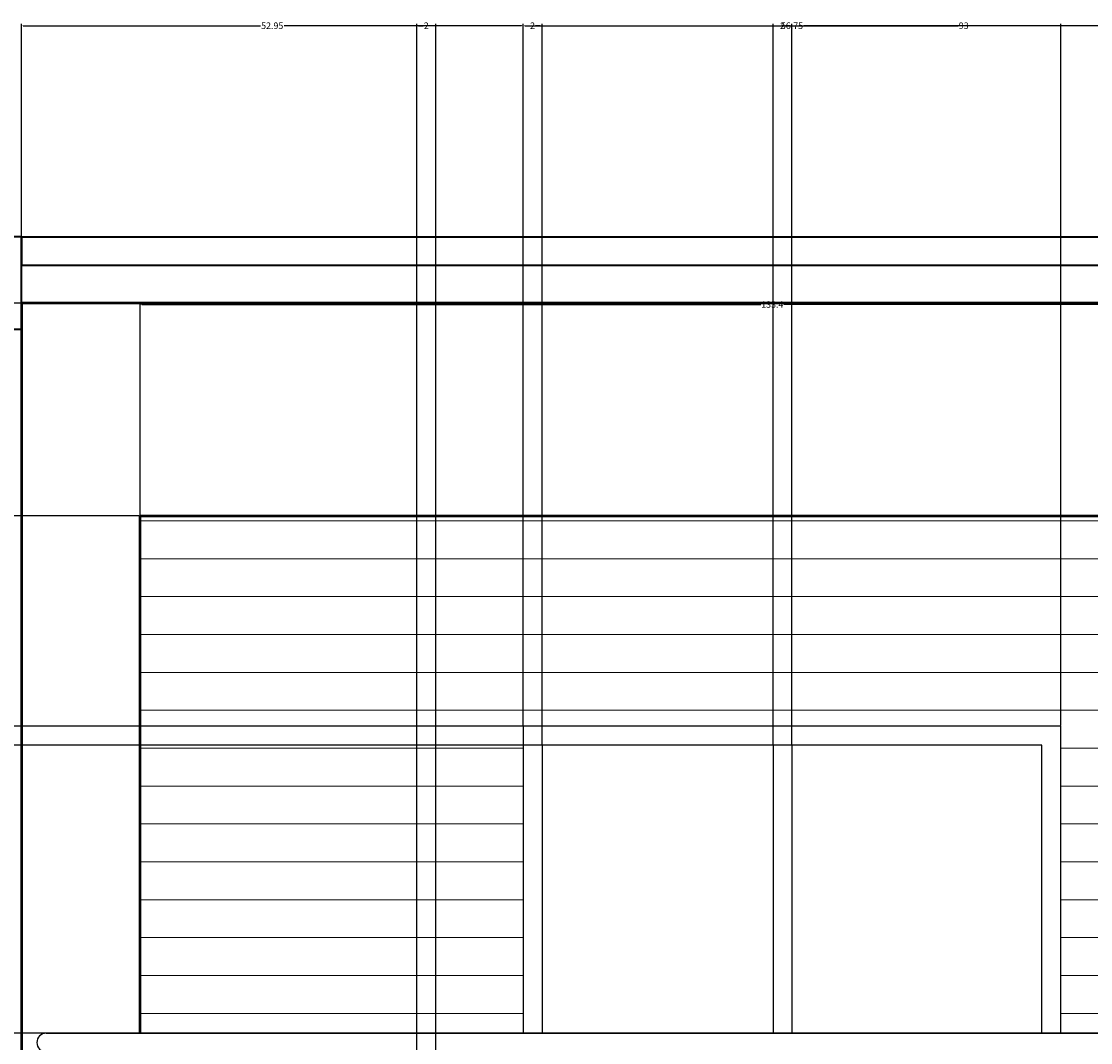
# Model space of a CAD drawing. Units: inches. Extents: x -139 to 346, y 72 to 413.
# Tile 8 of 18: x -47 to 66, y 305 to 413. Entities that reach past the tile are written whole.
import ezdxf

# ---------------------------------------------------------------- set-up
doc = ezdxf.new("R2010")
doc.units = ezdxf.units.IN
doc.header["$MEASUREMENT"] = 0
for name, color, linetype, lineweight in [('A-ANNO-DIMS', 2, 'Continuous', 18), ('A-DOOR', 3, 'Continuous', 25), ('A-ELEV-RAIL', 6, 'Continuous', 25), ('A-ROOF', 1, 'Continuous', 35), ('A-WALL', 7, 'Continuous', 50), ('A-WALL-PATT', 8, 'Continuous', 13)]:
    doc.layers.add(name, color=color, linetype=linetype, lineweight=lineweight)
doc.styles.get("Standard").update_dxf_attribs({"font": 'arial.ttf'})
doc.dimstyles.get("Standard").update_dxf_attribs({"dimtxt": 0.6875, "dimasz": 0.18, "dimexe": 0.18, "dimexo": 0.0625, "dimgap": 0.09, "dimtad": 0, "dimtih": 1, "dimtoh": 1, "dimdec": 4, "dimzin": 0, "dimdsep": 46, "dimlunit": 4, "dimtxsty": 'Standard', "dimcen": 0.09, "dimadec": 0, "dimazin": 0, "dimtfac": 1, "dimtdec": 4, "dimtofl": 0, "dimtmove": 0, "dimatfit": 3, "dimfxl": 1, "dimtolj": 1, "dimtzin": 0, "dimarcsym": 0})

# ---------------------------------------------------------------- blocks, each defined once
blk = doc.blocks.new('*D23')
at = {"layer": 'A-ANNO-DIMS', "color": 0, "lineweight": -2, "transparency": 16777216}
for p, q in [((-47.27, 383.04), (-47.27, 412.45)), ((-47.09, 412.27), (-22.05, 412.27)), ((5.49, 412.27), (-19.55, 412.27)), ((5.67, 338.38), (5.67, 412.45))]:
    blk.add_line(p, q, dxfattribs=at)
at = {"layer": 'A-ANNO-DIMS', "color": 0, "transparency": 16777216}
for points in [[(-47.09, 412.3), (-47.09, 412.24), (-47.27, 412.27)], [(5.49, 412.3), (5.49, 412.24), (5.67, 412.27)]]:
    blk.add_solid(points, dxfattribs=at)
at = {"layer": 'Defpoints', "color": 0, "transparency": 16777216}
for p in [(5.67, 412.27), (-47.27, 382.97), (5.67, 338.32)]:
    blk.add_point(p, dxfattribs=at)
at = {"layer": 'A-ANNO-DIMS', "color": 0, "transparency": 16777216, "insert": (-20.8, 412.27), "char_height": 0.688, "attachment_point": 5}
blk.add_mtext('\\A1;52.95', dxfattribs=at)
blk = doc.blocks.new('*D24')
at = {"layer": 'A-ANNO-DIMS', "color": 0, "lineweight": -2, "transparency": 16777216}
for p, q in [((5.67, 338.38), (5.67, 412.45)), ((5.85, 412.27), (32.8, 412.27)), ((62.25, 412.27), (35.3, 412.27)), ((62.43, 338.38), (62.43, 412.45))]:
    blk.add_line(p, q, dxfattribs=at)
at = {"layer": 'A-ANNO-DIMS', "color": 0, "transparency": 16777216}
for points in [[(5.85, 412.3), (5.85, 412.24), (5.67, 412.27)], [(62.25, 412.3), (62.25, 412.24), (62.43, 412.27)]]:
    blk.add_solid(points, dxfattribs=at)
at = {"layer": 'Defpoints', "color": 0, "transparency": 16777216}
for p in [(62.43, 412.27), (5.67, 338.32), (62.43, 338.32)]:
    blk.add_point(p, dxfattribs=at)
at = {"layer": 'A-ANNO-DIMS', "color": 0, "transparency": 16777216, "insert": (34.05, 412.27), "char_height": 0.688, "attachment_point": 5}
blk.add_mtext('\\A1;56.75', dxfattribs=at)
blk = doc.blocks.new('*D25')
at = {"layer": 'A-ANNO-DIMS', "color": 0, "lineweight": -2, "transparency": 16777216}
for p, q in [((5.67, 338.38), (5.67, 412.45)), ((5.85, 412.27), (51.59, 412.27)), ((98.49, 412.27), (52.76, 412.27)), ((98.67, 360.61), (98.67, 412.45))]:
    blk.add_line(p, q, dxfattribs=at)
at = {"layer": 'A-ANNO-DIMS', "color": 0, "transparency": 16777216}
for points in [[(5.85, 412.3), (5.85, 412.24), (5.67, 412.27)], [(98.49, 412.3), (98.49, 412.24), (98.67, 412.27)]]:
    blk.add_solid(points, dxfattribs=at)
at = {"layer": 'Defpoints', "color": 0, "transparency": 16777216}
for p in [(98.67, 412.27), (98.67, 360.54), (5.67, 338.32)]:
    blk.add_point(p, dxfattribs=at)
at = {"layer": 'A-ANNO-DIMS', "color": 0, "transparency": 16777216, "insert": (52.17, 412.27), "char_height": 0.688, "attachment_point": 5}
blk.add_mtext('\\A1;93', dxfattribs=at)
blk = doc.blocks.new('*D30')
at = {"layer": 'A-ANNO-DIMS', "color": 0, "lineweight": -2, "transparency": 16777216}
for p, q in [((-34.73, 360.61), (-34.73, 383.02)), ((-34.55, 382.84), (30.75, 382.84)), ((98.49, 382.84), (33.19, 382.84)), ((98.67, 360.61), (98.67, 383.02))]:
    blk.add_line(p, q, dxfattribs=at)
at = {"layer": 'A-ANNO-DIMS', "color": 0, "transparency": 16777216}
for points in [[(-34.55, 382.87), (-34.55, 382.81), (-34.73, 382.84)], [(98.49, 382.87), (98.49, 382.81), (98.67, 382.84)]]:
    blk.add_solid(points, dxfattribs=at)
at = {"layer": 'Defpoints', "color": 0, "transparency": 16777216}
for p in [(98.67, 382.84), (-34.73, 360.54), (98.67, 360.54)]:
    blk.add_point(p, dxfattribs=at)
at = {"layer": 'A-ANNO-DIMS', "color": 0, "transparency": 16777216, "insert": (31.97, 382.84), "char_height": 0.688, "attachment_point": 5}
blk.add_mtext('\\A1;133.4', dxfattribs=at)
blk = doc.blocks.new('*D44')
at = {"layer": 'A-ANNO-DIMS', "color": 0, "lineweight": -2, "transparency": 16777216}
for p, q in [((5.61, 338.32), (-137.3, 338.32)), ((-137.12, 338.14), (-137.12, 315.13)), ((-137.12, 291.24), (-137.12, 314.25)), ((-47.34, 291.06), (-137.3, 291.06))]:
    blk.add_line(p, q, dxfattribs=at)
at = {"layer": 'A-ANNO-DIMS', "color": 0, "transparency": 16777216}
for points in [[(-137.15, 338.14), (-137.09, 338.14), (-137.12, 338.32)], [(-137.15, 291.24), (-137.09, 291.24), (-137.12, 291.06)]]:
    blk.add_solid(points, dxfattribs=at)
at = {"layer": 'Defpoints', "color": 0, "transparency": 16777216}
for p in [(-137.12, 338.32), (5.67, 338.32), (-47.27, 291.06)]:
    blk.add_point(p, dxfattribs=at)
at = {"layer": 'A-ANNO-DIMS', "color": 0, "transparency": 16777216, "insert": (-137.12, 314.69), "char_height": 0.688, "attachment_point": 5}
blk.add_mtext('\\A1;47.26', dxfattribs=at)
blk = doc.blocks.new('*D45')
at = {"layer": 'A-ANNO-DIMS', "color": 0, "lineweight": -2, "transparency": 16777216}
for p, q in [((-34.8, 360.54), (-137.3, 360.54)), ((-137.12, 360.36), (-137.12, 349.87)), ((-137.12, 338.5), (-137.12, 348.99)), ((5.61, 338.32), (-137.3, 338.32))]:
    blk.add_line(p, q, dxfattribs=at)
at = {"layer": 'A-ANNO-DIMS', "color": 0, "transparency": 16777216}
for points in [[(-137.15, 360.36), (-137.09, 360.36), (-137.12, 360.54)], [(-137.15, 338.5), (-137.09, 338.5), (-137.12, 338.32)]]:
    blk.add_solid(points, dxfattribs=at)
at = {"layer": 'Defpoints', "color": 0, "transparency": 16777216}
for p in [(-137.12, 360.54), (-34.73, 360.54), (5.67, 338.32)]:
    blk.add_point(p, dxfattribs=at)
at = {"layer": 'A-ANNO-DIMS', "color": 0, "transparency": 16777216, "insert": (-137.12, 349.43), "char_height": 0.688, "attachment_point": 5}
blk.add_mtext('\\A1;22.223', dxfattribs=at)
blk = doc.blocks.new('*D46')
at = {"layer": 'A-ANNO-DIMS', "color": 0, "lineweight": -2, "transparency": 16777216}
for p, q in [((-47.34, 382.97), (-137.3, 382.97)), ((-137.12, 382.79), (-137.12, 372.2)), ((-137.12, 360.72), (-137.12, 371.32)), ((-34.8, 360.54), (-137.3, 360.54))]:
    blk.add_line(p, q, dxfattribs=at)
at = {"layer": 'A-ANNO-DIMS', "color": 0, "transparency": 16777216}
for points in [[(-137.15, 382.79), (-137.09, 382.79), (-137.12, 382.97)], [(-137.15, 360.72), (-137.09, 360.72), (-137.12, 360.54)]]:
    blk.add_solid(points, dxfattribs=at)
at = {"layer": 'Defpoints', "color": 0, "transparency": 16777216}
for p in [(-137.12, 382.97), (-47.27, 382.97), (-34.73, 360.54)]:
    blk.add_point(p, dxfattribs=at)
at = {"layer": 'A-ANNO-DIMS', "color": 0, "transparency": 16777216, "insert": (-137.12, 371.76), "char_height": 0.688, "attachment_point": 5}
blk.add_mtext('\\A1;22.43', dxfattribs=at)
blk = doc.blocks.new('*D68')
at = {"layer": 'A-ANNO-DIMS', "color": 0, "lineweight": -2, "transparency": 16777216}
for p, q in [((-5.54, 207.59), (-5.54, 412.45)), ((-5.36, 412.27), (-4.86, 412.27)), ((-3.72, 412.27), (-4.22, 412.27)), ((-3.54, 205.59), (-3.54, 412.45))]:
    blk.add_line(p, q, dxfattribs=at)
at = {"layer": 'A-ANNO-DIMS', "color": 0, "transparency": 16777216}
for points in [[(-5.36, 412.3), (-5.36, 412.24), (-5.54, 412.27)], [(-3.72, 412.3), (-3.72, 412.24), (-3.54, 412.27)]]:
    blk.add_solid(points, dxfattribs=at)
at = {"layer": 'Defpoints', "color": 0, "transparency": 16777216}
for p in [(-3.54, 412.27), (-5.54, 207.52), (-3.54, 205.52)]:
    blk.add_point(p, dxfattribs=at)
at = {"layer": 'A-ANNO-DIMS', "color": 0, "transparency": 16777216, "insert": (-4.54, 412.27), "char_height": 0.688, "attachment_point": 5}
blk.add_mtext('\\A1;2', dxfattribs=at)
blk = doc.blocks.new('*D89')
at = {"layer": 'A-ANNO-DIMS', "color": 0, "lineweight": -2, "transparency": 16777216}
for p, q in [((62.36, 338.32), (-137.3, 338.32)), ((-137.12, 338.14), (-137.12, 315.13)), ((-137.12, 291.24), (-137.12, 314.25)), ((62.36, 291.06), (-137.3, 291.06))]:
    blk.add_line(p, q, dxfattribs=at)
at = {"layer": 'A-ANNO-DIMS', "color": 0, "transparency": 16777216}
for points in [[(-137.15, 338.14), (-137.09, 338.14), (-137.12, 338.32)], [(-137.15, 291.24), (-137.09, 291.24), (-137.12, 291.06)]]:
    blk.add_solid(points, dxfattribs=at)
at = {"layer": 'Defpoints', "color": 0, "transparency": 16777216}
for p in [(-137.12, 338.32), (62.43, 338.32), (62.43, 291.06)]:
    blk.add_point(p, dxfattribs=at)
at = {"layer": 'A-ANNO-DIMS', "color": 0, "transparency": 16777216, "insert": (-137.12, 314.69), "char_height": 0.688, "attachment_point": 5}
blk.add_mtext('\\A1;47.26', dxfattribs=at)
blk = doc.blocks.new('*D90')
at = {"layer": 'A-ANNO-DIMS', "color": 0, "lineweight": -2, "transparency": 16777216}
for p, q in [((5.67, 338.38), (5.67, 412.45)), ((5.85, 412.27), (6.36, 412.27)), ((7.49, 412.27), (6.99, 412.27)), ((7.67, 336.38), (7.67, 412.45))]:
    blk.add_line(p, q, dxfattribs=at)
at = {"layer": 'A-ANNO-DIMS', "color": 0, "transparency": 16777216}
for points in [[(5.85, 412.3), (5.85, 412.24), (5.67, 412.27)], [(7.49, 412.3), (7.49, 412.24), (7.67, 412.27)]]:
    blk.add_solid(points, dxfattribs=at)
at = {"layer": 'Defpoints', "color": 0, "transparency": 16777216}
for p in [(7.67, 412.27), (5.67, 338.32), (7.67, 336.32)]:
    blk.add_point(p, dxfattribs=at)
at = {"layer": 'A-ANNO-DIMS', "color": 0, "transparency": 16777216, "insert": (6.67, 412.27), "char_height": 0.688, "attachment_point": 5}
blk.add_mtext('\\A1;2', dxfattribs=at)
blk = doc.blocks.new('*D91')
at = {"layer": 'A-ANNO-DIMS', "color": 0, "lineweight": -2, "transparency": 16777216}
for p, q in [((32.05, 336.38), (32.05, 412.45)), ((32.23, 412.27), (32.73, 412.27)), ((33.87, 412.27), (33.37, 412.27)), ((34.05, 336.38), (34.05, 412.45))]:
    blk.add_line(p, q, dxfattribs=at)
at = {"layer": 'A-ANNO-DIMS', "color": 0, "transparency": 16777216}
for points in [[(32.23, 412.3), (32.23, 412.24), (32.05, 412.27)], [(33.87, 412.3), (33.87, 412.24), (34.05, 412.27)]]:
    blk.add_solid(points, dxfattribs=at)
at = {"layer": 'Defpoints', "color": 0, "transparency": 16777216}
for p in [(34.05, 412.27), (32.05, 336.32), (34.05, 336.32)]:
    blk.add_point(p, dxfattribs=at)
at = {"layer": 'A-ANNO-DIMS', "color": 0, "transparency": 16777216, "insert": (33.05, 412.27), "char_height": 0.688, "attachment_point": 5}
blk.add_mtext('\\A1;2', dxfattribs=at)
blk = doc.blocks.new('*D92')
at = {"layer": 'A-ANNO-DIMS', "color": 0, "lineweight": -2, "transparency": 16777216}
for p, q in [((62.36, 338.32), (-137.3, 338.32)), ((-137.12, 338.14), (-137.12, 337.76)), ((60.36, 336.32), (-137.3, 336.32)), ((-137.12, 336.5), (-137.12, 336.89))]:
    blk.add_line(p, q, dxfattribs=at)
at = {"layer": 'A-ANNO-DIMS', "color": 0, "transparency": 16777216}
for points in [[(-137.15, 338.14), (-137.09, 338.14), (-137.12, 338.32)], [(-137.15, 336.5), (-137.09, 336.5), (-137.12, 336.32)]]:
    blk.add_solid(points, dxfattribs=at)
at = {"layer": 'Defpoints', "color": 0, "transparency": 16777216}
for p in [(62.43, 338.32), (-137.12, 336.32), (60.43, 336.32)]:
    blk.add_point(p, dxfattribs=at)
at = {"layer": 'A-ANNO-DIMS', "color": 0, "transparency": 16777216, "insert": (-137.12, 337.32), "char_height": 0.688, "attachment_point": 5}
blk.add_mtext('\\A1;2', dxfattribs=at)
blk = doc.blocks.new('*D100')
at = {"layer": 'A-ANNO-DIMS', "color": 0, "lineweight": -2, "transparency": 16777216}
for p, q in [((98.61, 305.92), (-137.3, 305.92)), ((-137.12, 305.74), (-137.12, 305.36)), ((98.61, 303.92), (-137.3, 303.92)), ((-137.12, 304.1), (-137.12, 304.49))]:
    blk.add_line(p, q, dxfattribs=at)
at = {"layer": 'A-ANNO-DIMS', "color": 0, "transparency": 16777216}
for points in [[(-137.15, 305.74), (-137.09, 305.74), (-137.12, 305.92)], [(-137.15, 304.1), (-137.09, 304.1), (-137.12, 303.92)]]:
    blk.add_solid(points, dxfattribs=at)
at = {"layer": 'Defpoints', "color": 0, "transparency": 16777216}
for p in [(-137.12, 305.92), (98.67, 305.92), (98.67, 303.92)]:
    blk.add_point(p, dxfattribs=at)
at = {"layer": 'A-ANNO-DIMS', "color": 0, "transparency": 16777216, "insert": (-137.12, 304.92), "char_height": 0.688, "attachment_point": 5}
blk.add_mtext('\\A1;2', dxfattribs=at)

msp = doc.modelspace()

# ---------------------------------------------------------------- hatches: boundary and pattern name
at = {"layer": 'A-WALL-PATT'}
h = msp.add_hatch(dxfattribs=at)
h.set_pattern_fill('ANSI31', color=256, scale=32, angle=135)
h.paths.add_polyline_path([(98.6724, 360.5443), (-34.7346, 360.5443), (-34.7346, 353.0644), (-34.7346, 305.9205), (5.6729, 305.9205), (5.6729, 338.3217), (62.4258, 338.3217), (62.4258, 305.9205), (98.6724, 305.9205)])
h.paths.add_polyline_path([(212.769, 231.0607), (175.072, 231.0607), (175.072, 218.0635), (171.0337, 218.0635), (171.0337, 115.6761), (125.2464, 115.6761), (125.2464, 218.0635), (123.4318, 218.0635), (120.5054, 218.0635), (120.5054, 231.0607), (112.6506, 231.0607), (112.6506, 112.6042), (212.769, 112.6042)])

# ---------------------------------------------------------------- linework, layer by layer
at = {"layer": 'A-DOOR'}
for p, q in [((32.0494, 336.3217), (32.0494, 305.9205)), ((34.0494, 336.3217), (34.0494, 305.9205))]:
    msp.add_line(p, q, dxfattribs=at)
for points in [[(62.4258, 305.9205), (62.4258, 338.3217), (5.6729, 338.3217), (5.6729, 305.9205)], [(60.4258, 305.9205), (60.4258, 336.3217), (7.6729, 336.3217), (7.6729, 305.9205)]]:
    msp.add_lwpolyline(points, dxfattribs=at)
at = {"layer": 'A-ELEV-RAIL'}
msp.add_line((-44.6423, 305.9205), (110.3243, 305.9205), dxfattribs=at)
msp.add_arc((-44.6423, 304.9205), 1, 90, 270, dxfattribs=at)
at = {"layer": 'A-ROOF'}
for p, q in [((-47.2734, 389.9748), (309.8894, 389.9748)), ((-47.2734, 389.9748), (-47.2734, 386.9748)), ((-47.2734, 382.9748), (-47.2734, 386.9748)), ((-47.2734, 386.9748), (309.8894, 386.9748))]:
    msp.add_line(p, q, dxfattribs=at)
msp.add_lwpolyline([(-47.2734, 389.9748), (-48.2494, 389.9748), (-48.2494, 380.2199), (-47.2734, 380.2199)], close=True, dxfattribs=at)
at = {"layer": 'A-WALL'}
for p, q in [((89.4597, 382.9748), (-47.2734, 382.9748)), ((-47.2734, 382.9748), (-47.2734, 291.0604)), ((-34.7346, 360.5443), (98.6724, 360.5443)), ((-34.7346, 353.0644), (-34.7346, 360.5443)), ((-34.7346, 305.9205), (-34.7346, 353.0644))]:
    msp.add_line(p, q, dxfattribs=at)

# ---------------------------------------------------------------- dimensions: what is measured, and where the dimension line sits
at = {"layer": 'A-ANNO-DIMS'}
for base, p1, p2, override, picture, middle in [((5.6729, 412.2748), (-47.2734, 382.9748), (5.6729, 338.3217), {"dimdec": 2, "dimlfac": 1, "dimrnd": 0, "dimzin": 0, "dimdsep": 46, "dimlunit": 2}, '*D23', (-20.8002, 412.2748)), ((-3.5402, 412.2748), (-5.5402, 207.5243), (-3.5402, 205.5243), {"dimdec": 0, "dimlfac": 1, "dimrnd": 0, "dimzin": 0, "dimdsep": 46, "dimlunit": 2}, '*D68', (-4.5402, 412.2748)), ((62.4258, 412.2748), (5.6729, 338.3217), (62.4258, 338.3217), {"dimdec": 2, "dimlfac": 1, "dimrnd": 0, "dimzin": 0, "dimdsep": 46, "dimlunit": 2}, '*D24', (34.0494, 412.2748)), ((98.6724, 412.2748), (5.6729, 338.3217), (98.6724, 360.5443), {"dimdec": 0, "dimlfac": 1, "dimrnd": 0, "dimzin": 0, "dimdsep": 46, "dimlunit": 2}, '*D25', (52.1727, 412.2748)), ((7.6729, 412.2748), (5.6729, 338.3217), (7.6729, 336.3217), {"dimdec": 0, "dimlfac": 1, "dimrnd": 0, "dimzin": 0, "dimdsep": 46, "dimlunit": 2}, '*D90', (6.6729, 412.2748)), ((34.0494, 412.2748), (32.0494, 336.3217), (34.0494, 336.3217), {"dimdec": 0, "dimlfac": 1, "dimrnd": 0, "dimzin": 0, "dimdsep": 46, "dimlunit": 2}, '*D91', (33.0494, 412.2748)), ((98.6724, 382.8443), (-34.7346, 360.5443), (98.6724, 360.5443), {"dimdec": 1, "dimlfac": 1, "dimrnd": 0, "dimzin": 0, "dimdsep": 46, "dimlunit": 2}, '*D30', (31.9689, 382.8443))]:
    dim = msp.add_linear_dim(base=base, p1=p1, p2=p2, dimstyle='Standard', override=override, dxfattribs=at)
    dim.commit()
    dim.dimension.update_dxf_attribs({"geometry": picture, "text_midpoint": middle})
for base, p1, p2, override, picture, middle in [((-137.1237, 382.9748), (-34.7346, 360.5443), (-47.2734, 382.9748), {"dimdec": 2, "dimlfac": 1, "dimrnd": 0, "dimzin": 0, "dimdsep": 46, "dimlunit": 2}, '*D46', (-137.1237, 371.7595)), ((-137.1237, 360.5443), (5.6729, 338.3217), (-34.7346, 360.5443), {"dimdec": 3, "dimlfac": 1, "dimrnd": 0, "dimzin": 0, "dimdsep": 46, "dimlunit": 2}, '*D45', (-137.1237, 349.433)), ((-137.1237, 338.3217), (-47.2734, 291.0604), (5.6729, 338.3217), {"dimdec": 2, "dimlfac": 1, "dimrnd": 0, "dimzin": 0, "dimdsep": 46, "dimlunit": 2}, '*D44', (-137.1237, 314.691)), ((-137.1237, 338.3217), (62.4258, 291.0604), (62.4258, 338.3217), {"dimdec": 2, "dimlfac": 1, "dimrnd": 0, "dimzin": 0, "dimdsep": 46, "dimlunit": 2}, '*D89', (-137.1237, 314.691)), ((-137.1237, 336.3217), (62.4258, 338.3217), (60.4258, 336.3217), {"dimdec": 0, "dimlfac": 1, "dimrnd": 0, "dimzin": 0, "dimdsep": 46, "dimlunit": 2}, '*D92', (-137.1237, 337.3217)), ((-137.1237, 305.9205), (98.6724, 303.9205), (98.6724, 305.9205), {"dimdec": 0, "dimlfac": 1, "dimrnd": 0, "dimzin": 0, "dimdsep": 46, "dimlunit": 2}, '*D100', (-137.1237, 304.9205))]:
    dim = msp.add_linear_dim(base=base, p1=p1, p2=p2, angle=90, dimstyle='Standard', override=override, dxfattribs=at)
    dim.commit()
    dim.dimension.update_dxf_attribs({"geometry": picture, "text_midpoint": middle})

doc.saveas('drawing.dxf')
